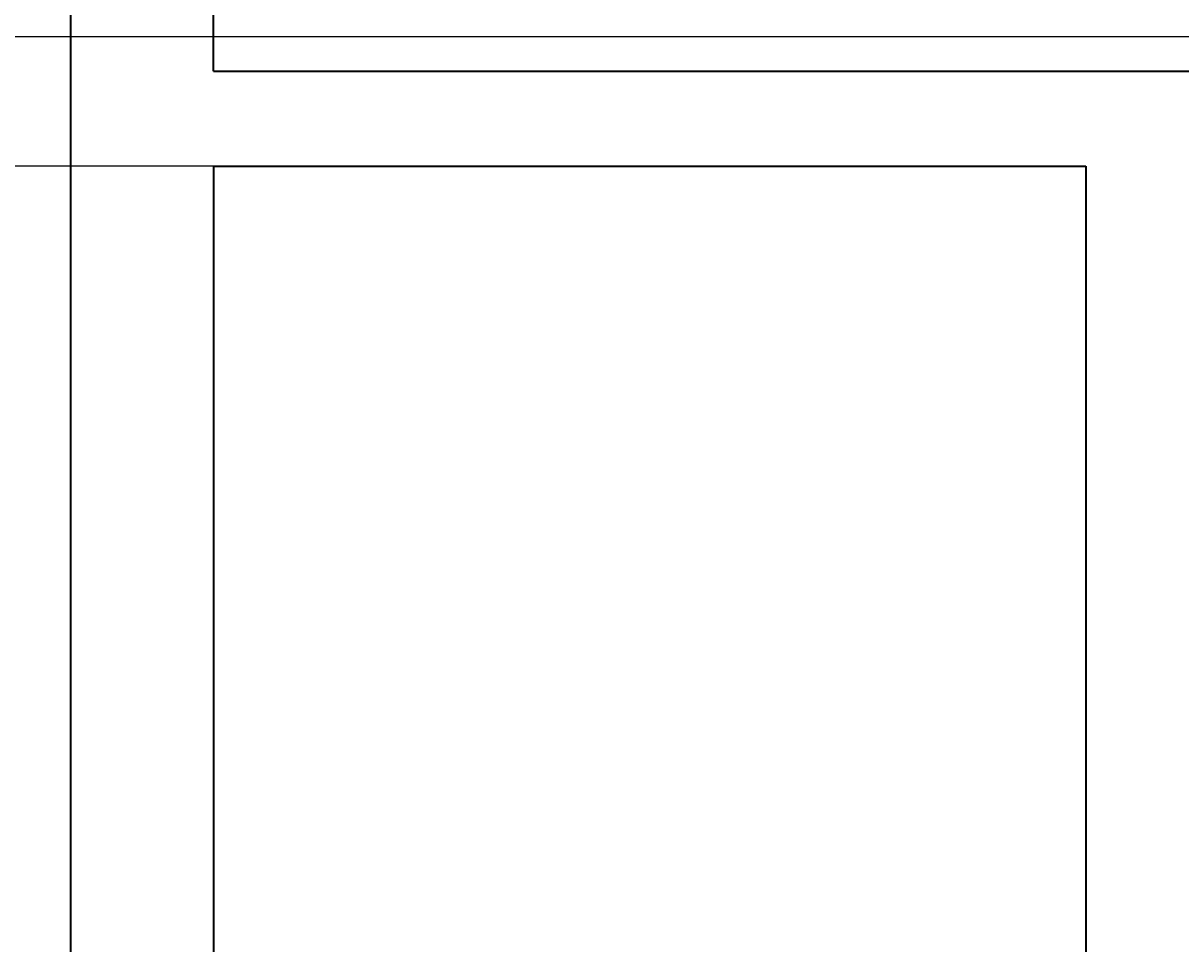
# Model space of a CAD drawing. Units: inches. Extents: x -61 to 1599, y -1316 to 257.
# Tile 59 of 204: x 12 to 85, y -224 to -166. Entities that reach past the tile are written whole.
import ezdxf

# ---------------------------------------------------------------- set-up
doc = ezdxf.new("R2010")
doc.units = ezdxf.units.IN
doc.header["$MEASUREMENT"] = 0
doc.layers.add('A-ANNO-DIMS', color=2, linetype='Continuous', lineweight=18)
doc.layers.add('WALLS', color=4, linetype='Continuous', lineweight=35)
doc.styles.get("Standard").update_dxf_attribs({"font": 'arial.ttf'})
doc.dimstyles.get("Standard").update_dxf_attribs({"dimtxt": 0.18, "dimasz": 0.18, "dimexe": 0.18, "dimexo": 0.0625, "dimgap": 0.09, "dimtad": 0, "dimtih": 1, "dimtoh": 1, "dimdec": 0, "dimzin": 0, "dimdsep": 46, "dimlunit": 3, "dimtxsty": 'Standard', "dimcen": 0.09, "dimadec": 0, "dimazin": 0, "dimtfac": 1, "dimtdec": 0, "dimtofl": 0, "dimtmove": 0, "dimatfit": 3, "dimfxl": 1, "dimtolj": 1, "dimtzin": 0, "dimarcsym": 0})

# ---------------------------------------------------------------- blocks, each defined once
blk = doc.blocks.new('*D687')
at = {"layer": 'A-ANNO-DIMS', "color": 0, "lineweight": -2, "transparency": 16777216}
for p, q in [((289.418, 181.677), (-61.077, 181.677)), ((-60.897, 181.497), (-60.897, -528.952)), ((-60.897, -1239.765), (-60.897, -529.316)), ((319.64, -1239.945), (-61.077, -1239.945))]:
    blk.add_line(p, q, dxfattribs=at)
at = {"layer": 'A-ANNO-DIMS', "color": 0, "transparency": 16777216}
for points in [[(-60.927, 181.497), (-60.867, 181.497), (-60.897, 181.677)], [(-60.927, -1239.765), (-60.867, -1239.765), (-60.897, -1239.945)]]:
    blk.add_solid(points, dxfattribs=at)
at = {"layer": 'DEFPOINTS', "color": 0, "transparency": 16777216}
for p in [(289.481, 181.677), (-60.897, -1239.945), (319.703, -1239.945)]:
    blk.add_point(p, dxfattribs=at)
at = {"layer": 'A-ANNO-DIMS', "color": 0, "transparency": 16777216, "insert": (-60.897, -529.134), "char_height": 0.18, "attachment_point": 5}
blk.add_mtext('\\A1;1421.6', dxfattribs=at)
blk = doc.blocks.new('*D691')
at = {"layer": 'A-ANNO-DIMS', "color": 0, "lineweight": -2, "transparency": 16777216}
for p, q in [((14.64, 157.677), (-61.077, 157.677)), ((-60.897, 157.497), (-60.897, -141.641)), ((-60.897, -441.143), (-60.897, -142.005)), ((14.64, -441.323), (-61.077, -441.323))]:
    blk.add_line(p, q, dxfattribs=at)
at = {"layer": 'A-ANNO-DIMS', "color": 0, "transparency": 16777216}
for points in [[(-60.927, 157.497), (-60.867, 157.497), (-60.897, 157.677)], [(-60.927, -441.143), (-60.867, -441.143), (-60.897, -441.323)]]:
    blk.add_solid(points, dxfattribs=at)
at = {"layer": 'DEFPOINTS', "color": 0, "transparency": 16777216}
for p in [(-60.897, 157.677), (14.703, 157.677), (14.703, -441.323)]:
    blk.add_point(p, dxfattribs=at)
at = {"layer": 'A-ANNO-DIMS', "color": 0, "transparency": 16777216, "insert": (-60.897, -141.823), "char_height": 0.18, "attachment_point": 5}
blk.add_mtext('\\A1;599', dxfattribs=at)
blk = doc.blocks.new('*D699')
at = {"layer": 'A-ANNO-DIMS', "color": 0, "lineweight": -2, "transparency": 16777216}
for p, q in [((835.64, -167.169), (-61.077, -167.169)), ((-60.897, -167.349), (-60.897, -306.726)), ((-60.897, -446.466), (-60.897, -307.09)), ((841.64, -446.646), (-61.077, -446.646))]:
    blk.add_line(p, q, dxfattribs=at)
at = {"layer": 'A-ANNO-DIMS', "color": 0, "transparency": 16777216}
for points in [[(-60.927, -167.349), (-60.867, -167.349), (-60.897, -167.169)], [(-60.927, -446.466), (-60.867, -446.466), (-60.897, -446.646)]]:
    blk.add_solid(points, dxfattribs=at)
at = {"layer": 'DEFPOINTS', "color": 0, "transparency": 16777216}
for p in [(835.703, -167.169), (-60.897, -446.646), (841.703, -446.646)]:
    blk.add_point(p, dxfattribs=at)
at = {"layer": 'A-ANNO-DIMS', "color": 0, "transparency": 16777216, "insert": (-60.897, -306.908), "char_height": 0.18, "attachment_point": 5}
blk.add_mtext('\\A1;279.5', dxfattribs=at)
blk = doc.blocks.new('*D700')
at = {"layer": 'A-ANNO-DIMS', "color": 0, "lineweight": -2, "transparency": 16777216}
for p, q in [((14.703, -616.882), (14.703, 257.457)), ((14.883, 257.277), (96.772, 257.277)), ((179.572, 257.277), (97.683, 257.277)), ((179.752, -616.882), (179.752, 257.457))]:
    blk.add_line(p, q, dxfattribs=at)
at = {"layer": 'A-ANNO-DIMS', "color": 0, "transparency": 16777216}
for points in [[(14.883, 257.307), (14.883, 257.247), (14.703, 257.277)], [(179.572, 257.307), (179.572, 257.247), (179.752, 257.277)]]:
    blk.add_solid(points, dxfattribs=at)
at = {"layer": 'DEFPOINTS', "color": 0, "transparency": 16777216}
for p in [(179.752, 257.277), (14.703, -616.945), (179.752, -616.945)]:
    blk.add_point(p, dxfattribs=at)
at = {"layer": 'A-ANNO-DIMS', "color": 0, "transparency": 16777216, "insert": (97.227, 257.277), "char_height": 0.18, "attachment_point": 5}
blk.add_mtext('\\A1;165.05', dxfattribs=at)
blk = doc.blocks.new('*D706')
at = {"layer": 'A-ANNO-DIMS', "color": 0, "lineweight": -2, "transparency": 16777216}
for p, q in [((78.64, -175.323), (-61.077, -175.323)), ((-60.897, -175.503), (-60.897, -212.976)), ((-60.897, -250.814), (-60.897, -213.34)), ((78.64, -250.994), (-61.077, -250.994))]:
    blk.add_line(p, q, dxfattribs=at)
at = {"layer": 'A-ANNO-DIMS', "color": 0, "transparency": 16777216}
for points in [[(-60.927, -175.503), (-60.867, -175.503), (-60.897, -175.323)], [(-60.927, -250.814), (-60.867, -250.814), (-60.897, -250.994)]]:
    blk.add_solid(points, dxfattribs=at)
at = {"layer": 'DEFPOINTS', "color": 0, "transparency": 16777216}
for p in [(-60.897, -175.323), (78.703, -175.323), (78.703, -250.994)]:
    blk.add_point(p, dxfattribs=at)
at = {"layer": 'A-ANNO-DIMS', "color": 0, "transparency": 16777216, "insert": (-60.897, -213.158), "char_height": 0.18, "attachment_point": 5}
blk.add_mtext('\\A1;75.67', dxfattribs=at)

msp = doc.modelspace()

# ---------------------------------------------------------------- linework, layer by layer
at = {"layer": 'WALLS'}
for p, q in [((14.7028, 157.6771), (14.7028, -441.3229)), ((23.7028, -169.3229), (23.7028, -13.3229)), ((23.7028, -169.3229), (113.7028, -169.3229)), ((23.7028, -175.3229), (78.7028, -175.3229)), ((23.7028, -175.3229), (23.7028, -432.3229)), ((78.7028, -175.3229), (78.7028, -432.3229))]:
    msp.add_line(p, q, dxfattribs=at)

# ---------------------------------------------------------------- dimensions: what is measured, and where the dimension line sits
at = {"layer": 'A-ANNO-DIMS'}
dim = msp.add_linear_dim(base=(179.7521, 257.2771), p1=(14.7028, -616.9446), p2=(179.7521, -616.9446), dimstyle='Standard', override={"dimdec": 2, "dimlfac": 1, "dimrnd": 0, "dimzin": 0, "dimdsep": 46, "dimlunit": 2}, dxfattribs=at)
dim.commit()
dim.dimension.update_dxf_attribs({"geometry": '*D700', "text_midpoint": (97.2274, 257.2771)})
for base, p1, p2, override, picture, middle in [((-60.8972, -1239.9446), (289.4807, 181.6771), (319.7028, -1239.9446), {"dimdec": 1, "dimlfac": 1, "dimrnd": 0, "dimzin": 0, "dimdsep": 46, "dimlunit": 2}, '*D687', (-60.8972, -529.1337)), ((-60.8972, 157.6771), (14.7028, -441.3229), (14.7028, 157.6771), {"dimdec": 0, "dimlfac": 1, "dimrnd": 0, "dimzin": 0, "dimdsep": 46, "dimlunit": 2}, '*D691', (-60.8972, -141.8229)), ((-60.8972, -446.6462), (835.7028, -167.169), (841.7028, -446.6462), {"dimdec": 1, "dimlfac": 1, "dimrnd": 0, "dimzin": 0, "dimdsep": 46, "dimlunit": 2}, '*D699', (-60.8972, -306.9076)), ((-60.8972, -175.3229), (78.7028, -250.9938), (78.7028, -175.3229), {"dimdec": 2, "dimlfac": 1, "dimrnd": 0, "dimzin": 0, "dimdsep": 46, "dimlunit": 2}, '*D706', (-60.8972, -213.1583))]:
    dim = msp.add_linear_dim(base=base, p1=p1, p2=p2, angle=90, dimstyle='Standard', override=override, dxfattribs=at)
    dim.commit()
    dim.dimension.update_dxf_attribs({"geometry": picture, "text_midpoint": middle})

doc.saveas('drawing.dxf')
